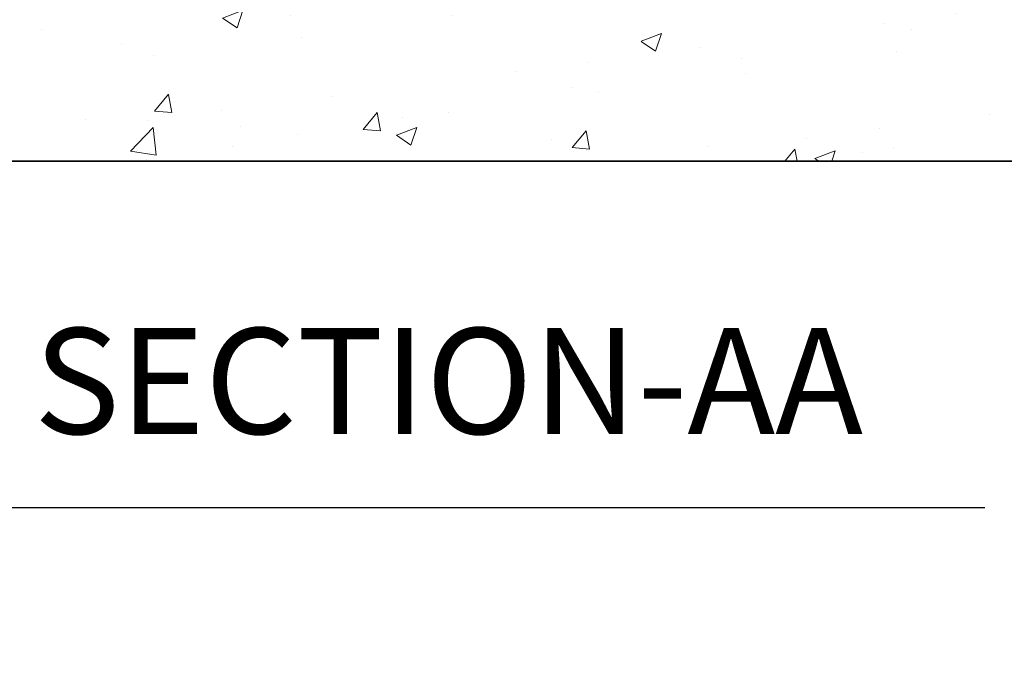
# Model space of a CAD drawing. Units: inches. Extents: x 2416 to 3391, y 1375 to 2496.
# Tile 6 of 13: x 2994 to 3105, y 2069 to 2142. Entities that reach past the tile are written whole.
import ezdxf

# ---------------------------------------------------------------- set-up
doc = ezdxf.new("R2010")
doc.units = ezdxf.units.IN
for name, color, linetype, lineweight in [('A-ANNO-DIMS', 2, 'Continuous', 18), ('A-ANNO-TITL', 7, 'Continuous', 30), ('A-FLOR-PATT', 252, 'Continuous', 13), ('A-SECT', 7, 'Continuous', 35)]:
    doc.layers.add(name, color=color, linetype=linetype, lineweight=lineweight)
doc.styles.get("Standard").update_dxf_attribs({"font": 'arial.ttf'})
doc.dimstyles.get("Standard").update_dxf_attribs({"dimtxt": 0.18, "dimasz": 0.18, "dimexe": 0.18, "dimexo": 0.0625, "dimgap": 0.09, "dimtad": 0, "dimtih": 1, "dimtoh": 1, "dimdec": 4, "dimzin": 0, "dimdsep": 46, "dimtxsty": 'Standard', "dimcen": 0.09, "dimadec": 0, "dimazin": 0, "dimtfac": 1, "dimtdec": 4, "dimtofl": 0, "dimtmove": 0, "dimatfit": 3, "dimfxl": 1, "dimtolj": 1, "dimtzin": 0, "dimarcsym": 0})

# ---------------------------------------------------------------- blocks, each defined once
blk = doc.blocks.new('*D83')
at = {"layer": 'A-ANNO-DIMS', "color": 0, "lineweight": -2, "transparency": 16777216}
for p, q in [((2904.19, 2125.8), (2904.19, 2062.03)), ((3202.69, 2125.8), (3202.69, 2062.03)), ((2904.37, 2062.21), (3053.05, 2062.21)), ((3202.51, 2062.21), (3053.84, 2062.21))]:
    blk.add_line(p, q, dxfattribs=at)
at = {"layer": 'A-ANNO-DIMS', "color": 0, "transparency": 16777216}
for points in [[(2904.37, 2062.24), (2904.37, 2062.18), (2904.19, 2062.21)], [(3202.51, 2062.24), (3202.51, 2062.18), (3202.69, 2062.21)]]:
    blk.add_solid(points, dxfattribs=at)
at = {"layer": 'Defpoints', "color": 0, "transparency": 16777216}
for p in [(2904.19, 2125.86), (3202.69, 2125.86), (3202.69, 2062.21)]:
    blk.add_point(p, dxfattribs=at)
at = {"layer": 'A-ANNO-DIMS', "color": 0, "transparency": 16777216, "insert": (3053.44, 2062.21), "char_height": 0.18, "attachment_point": 5}
blk.add_mtext('\\A1;298.5', dxfattribs=at)

msp = doc.modelspace()

# ---------------------------------------------------------------- hatches: boundary and pattern name
at = {"layer": 'A-FLOR-PATT'}
h = msp.add_hatch(dxfattribs=at)
h.set_pattern_fill('AR-CONC', color=256, scale=0.13, style=0)
h.paths.add_polyline_path([(2904.1924, 2125.8608), (3202.6924, 2125.8608), (3202.6924, 2143.8608), (2904.1924, 2143.8608)])

# ---------------------------------------------------------------- linework, layer by layer
at = {"layer": 'A-ANNO-TITL'}
msp.add_line((2987.8706, 2086.6125), (3103.051, 2086.6125), dxfattribs=at)
at = {"layer": 'A-SECT'}
msp.add_line((3202.6924, 2125.8608), (2904.1924, 2125.8608), dxfattribs=at)

# ---------------------------------------------------------------- texts
at = {"layer": 'A-ANNO-TITL', "insert": (2995.2133, 2106.952), "char_height": 12, "attachment_point": 1}
msp.add_mtext_dynamic_manual_height_columns('SECTION-AA', width=198.936669, gutter_width=12.5, heights=[0], dxfattribs=at)

# ---------------------------------------------------------------- dimensions: what is measured, and where the dimension line sits
at = {"layer": 'A-ANNO-DIMS'}
dim = msp.add_linear_dim(base=(3202.6924, 2062.2125), p1=(2904.1924, 2125.8608), p2=(3202.6924, 2125.8608), dimstyle='Standard', override={"dimdec": 1, "dimlfac": 1, "dimrnd": 0, "dimzin": 0, "dimdsep": 46, "dimlunit": 2}, dxfattribs=at)
dim.commit()
dim.dimension.update_dxf_attribs({"geometry": '*D83', "text_midpoint": (3053.4424, 2062.2125)})

doc.saveas('drawing.dxf')
